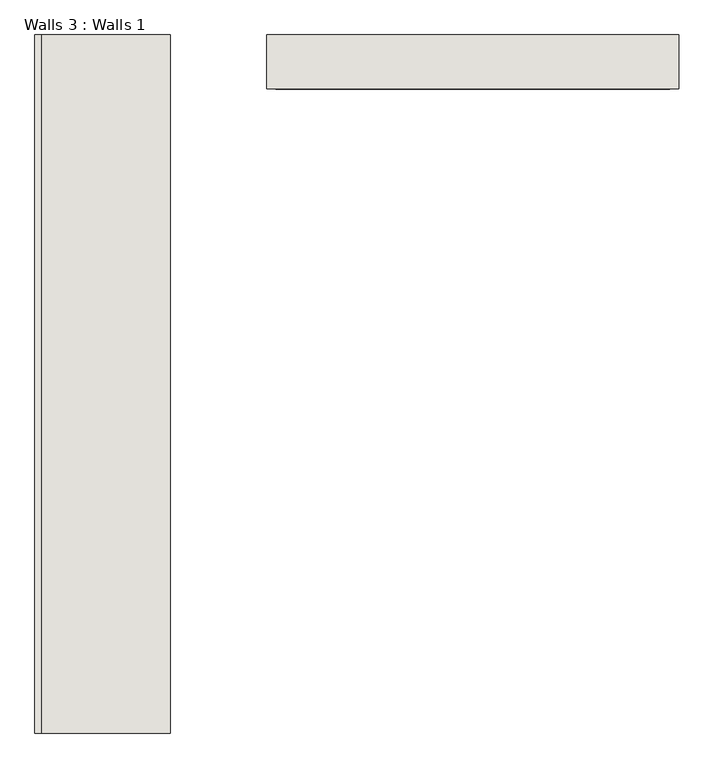
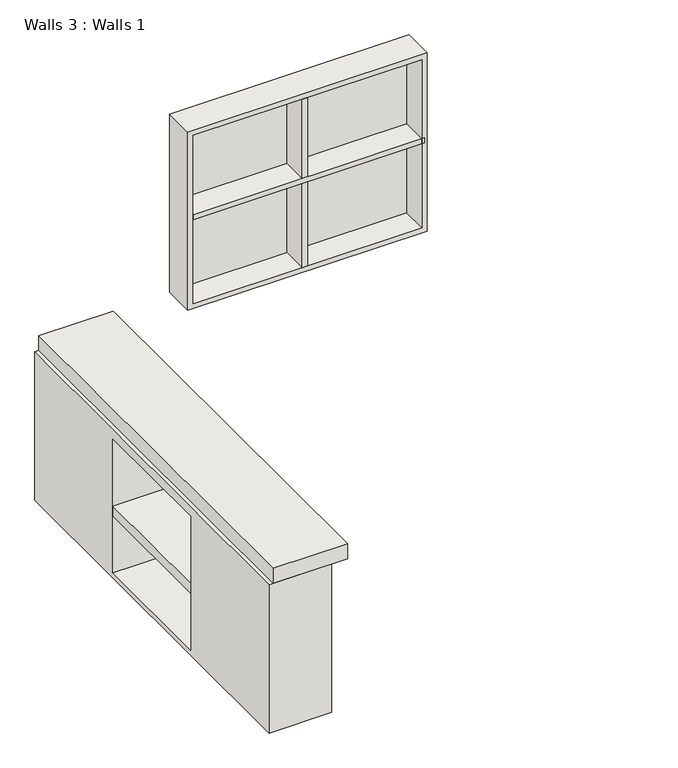
"""IFC4 building model written with IfcOpenShell, lengths in millimetres: wall geometry, Walls 3 : Walls 1."""

from ifc_helpers import new_model, si_unit, frame, origin, place, context, project, spatial, polyline, outline, extrude, faceted_brep, source, transform, mapped, element, save


def walls_3_walls_1_7bd47e67(model_context):
    return source(origin(), model_context, "Body", "SolidModel", [
        extrude(outline(polyline([(-4669.7681702, -2647.557676), (-4669.7681702, -2774.557676), (-5793.7181702, -2774.557676), (-5793.7181702, -2647.557676), (-4669.7681702, -2647.557676)])), frame((0.0, 0.0, 4522.8031259), z_axis=(0.0, 0.0, 1.0), x_axis=(1.0, 0.0, 0.0)), (0.0, 0.0, 1.0), 25.4),
        extrude(outline(polyline([(-5263.4931702, -2774.557676), (-5263.4931702, -2647.557676), (-5238.0931702, -2647.557676), (-5238.0931702, -2774.557676), (-5263.4931702, -2774.557676)])), frame((0.0, 0.0, 4091.0031259), z_axis=(0.0, 0.0, 1.0), x_axis=(1.0, 0.0, 0.0)), (0.0, 0.0, 1.0), 863.6),
        faceted_brep([(-4657.0681702, -2774.557676, 4065.6031259), (-4657.0681702, -2774.557676, 4980.0031259), (-5819.1181702, -2774.557676, 4980.0031259), (-5819.1181702, -2774.557676, 4065.6031259), (-4682.4681702, -2774.557676, 4954.6031259), (-4682.4681702, -2774.557676, 4091.0031259), (-5793.7181702, -2774.557676, 4091.0031259), (-5793.7181702, -2774.557676, 4954.6031259), (-4657.0681702, -2622.157676, 4065.6031259), (-5819.1181702, -2622.157676, 4065.6031259), (-5819.1181702, -2622.157676, 4980.0031259), (-4657.0681702, -2622.157676, 4980.0031259), (-4682.4681702, -2647.557676, 4954.6031259), (-5793.7181702, -2647.557676, 4954.6031259), (-5793.7181702, -2647.557676, 4091.0031259), (-4682.4681702, -2647.557676, 4091.0031259)], [[[0, 1, 2, 3], [4, 5, 6, 7]], [[8, 9, 10, 11]], [[1, 0, 8, 11]], [[2, 1, 11, 10]], [[3, 2, 10, 9]], [[0, 3, 9, 8]], [[12, 13, 14, 15]], [[12, 15, 5, 4]], [[15, 14, 6, 5]], [[14, 13, 7, 6]], [[13, 12, 4, 7]]]),
        extrude(outline(polyline([(-6454.1181702, -2622.157676), (-6092.1681702, -2622.157676), (-6092.1681702, -4590.657676), (-6454.1181702, -4590.657676), (-6454.1181702, -2622.157676)])), frame((0.0, 0.0, 3989.4031259), z_axis=(0.0, 0.0, 1.0), x_axis=(1.0, 0.0, 0.0)), (0.0, 0.0, 1.0), 76.2),
        extrude(outline(polyline([(-6165.8877015, -3282.4431283), (-6165.8877015, -3592.120176), (-6170.9478577, -3592.120176), (-6170.9478577, -3282.4431283), (-6165.8877015, -3282.4431283)])), frame((0.0, 0.0, 3245.9519176), z_axis=(0.0, 0.0, 1.0), x_axis=(1.0, 0.0, 0.0)), (0.0, 0.0, 1.0), 685.8),
        extrude(outline(polyline([(-6163.308014, -3603.6829064), (-6163.308014, -3930.257676), (-6168.3681702, -3930.257676), (-6168.3681702, -3603.6829064), (-6163.308014, -3603.6829064)])), frame((0.0, 0.0, 3252.8031259), z_axis=(0.0, 0.0, 1.0), x_axis=(1.0, 0.0, 0.0)), (0.0, 0.0, 1.0), 685.8),
        extrude(outline(polyline([(-6168.3681702, -3277.1081367), (-6168.3681702, -3930.257676), (-6473.1681702, -3930.257676), (-6473.1681702, -3277.1081367), (-6168.3681702, -3277.1081367)])), frame((0.0, 0.0, 3544.9031259), z_axis=(0.0, 0.0, 1.0), x_axis=(1.0, 0.0, 0.0)), (0.0, 0.0, 1.0), 50.8),
        extrude(outline(polyline([(-2622.157676, 3227.4031259), (-4590.657676, 3227.4031259), (-4590.657676, 3989.4031259), (-2622.157676, 3989.4031259), (-2622.157676, 3227.4031259)]), holes=[polyline([(-3277.1081367, 3252.8031259), (-3277.1081367, 3938.6031259), (-3930.257676, 3938.6031259), (-3930.257676, 3252.8031259), (-3277.1081367, 3252.8031259)])]), frame((-6473.1681702, 0.0, 0.0), z_axis=(1.0, 0.0, 0.0), x_axis=(0.0, 1.0, 0.0)), (0.0, 0.0, 1.0), 304.8),
        extrude(outline(polyline([(-6165.7884827, -2647.557676), (-6165.7884827, -3257.157676), (-6168.3681702, -3257.157676), (-6168.3681702, -2647.557676), (-6165.7884827, -2647.557676)])), frame((0.0, 0.0, 3255.9781259), z_axis=(0.0, 0.0, 1.0), x_axis=(1.0, 0.0, 0.0)), (0.0, 0.0, 1.0), 298.45),
        extrude(outline(polyline([(-6165.7884827, -2647.557676), (-6165.7884827, -3257.157676), (-6168.3681702, -3257.157676), (-6168.3681702, -2647.557676), (-6165.7884827, -2647.557676)])), frame((0.0, 0.0, 3598.2431259), z_axis=(0.0, 0.0, 1.0), x_axis=(1.0, 0.0, 0.0)), (0.0, 0.0, 1.0), 365.76),
        extrude(outline(polyline([(-6165.7884827, -3955.657676), (-6165.7884827, -4565.257676), (-6168.3681702, -4565.257676), (-6168.3681702, -3955.657676), (-6165.7884827, -3955.657676)])), frame((0.0, 0.0, 3255.9781259), z_axis=(0.0, 0.0, 1.0), x_axis=(1.0, 0.0, 0.0)), (0.0, 0.0, 1.0), 298.45),
        extrude(outline(polyline([(-6165.7884827, -3955.657676), (-6165.7884827, -4565.257676), (-6168.3681702, -4565.257676), (-6168.3681702, -3955.657676), (-6165.7884827, -3955.657676)])), frame((0.0, 0.0, 3598.2431259), z_axis=(0.0, 0.0, 1.0), x_axis=(1.0, 0.0, 0.0)), (0.0, 0.0, 1.0), 365.76),
    ])


if __name__ == "__main__":
    model = new_model("IFC4")
    model_context = context("Model", 3, world=origin())
    ifc_project = project(units=[si_unit("LENGTHUNIT", "METRE", prefix="MILLI")], contexts=[model_context])
    site = spatial("IfcSite", under=ifc_project)
    building = spatial("IfcBuilding", under=site)
    placement = place(None, origin())
    walls_3_walls_1_shape = walls_3_walls_1_7bd47e67(model_context)
    element("IfcWall", 1, ObjectType="Walls 3 : Walls 1", at=placement, inside=building, context=model_context, shape_type="MappedRepresentation", body=[
        mapped(walls_3_walls_1_shape, transform((0.0, 0.0, 0.0), x_axis=(1.0, 0.0, 0.0), y_axis=(0.0, 1.0, 0.0), z_axis=(0.0, 0.0, 1.0))),
    ])
    save(model, "model.ifc")

# Revit data of these elements
# Element 1 (IfcWall, "Walls 3 : Walls 1")
#   Materials on its faces: "drawers", "wood", "clear glass", "stone", "Default Wall"
# Materials
#   "drawers": class "Generic", colour RGB 121 66 39, transparency 0, Cost = 0
#   "wood": class "Generic", colour RGB 255 226 181, transparency 0, Cost = 0
#   "clear glass": class "Generic", colour RGB 141 181 235, transparency 0.9, Cost = 0
#   "stone": class "Generic", colour RGB 125 126 130, transparency 0, Cost = 0
#   "Default Wall": colour RGB 128 128 128, transparency 0
